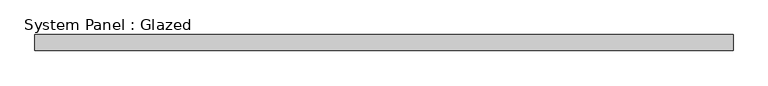
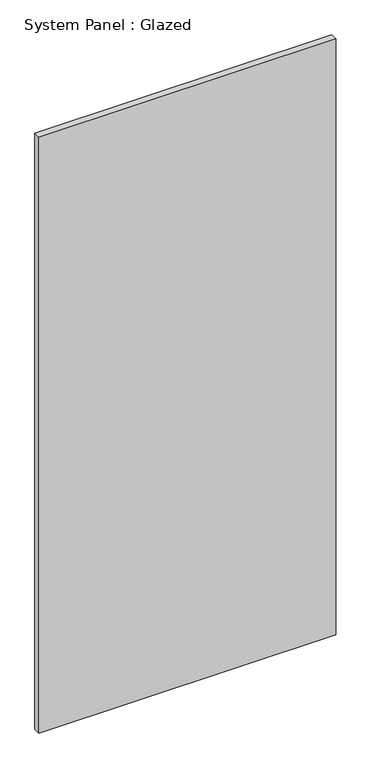
"""IFC4 building model written with IfcOpenShell, lengths in millimetres: plate geometry, System Panel : Glazed."""

from ifc_helpers import new_model, si_unit, origin, origin_with_axes, place, context, project, spatial, polyline, outline, extrude, source, transform, mapped, element, save


def system_panel_glazed_87980334(model_context):
    return source(origin(), model_context, "Body", "SweptSolid", [
        extrude(outline(polyline([(552.4499999, 19.05), (-552.4499999, 19.05), (-552.4499999, 44.45), (552.4499999, 44.45), (552.4499999, 19.05)])), origin_with_axes(), (0.0, 0.0, 1.0), 2343.15),
    ])


if __name__ == "__main__":
    model = new_model("IFC4")
    model_context = context("Model", 3, world=origin())
    ifc_project = project(units=[si_unit("LENGTHUNIT", "METRE", prefix="MILLI")], contexts=[model_context])
    site = spatial("IfcSite", under=ifc_project)
    building = spatial("IfcBuilding", under=site)
    placement = place(None, origin())
    system_panel_glazed_shape = system_panel_glazed_87980334(model_context)
    element("IfcPlate", 1, ObjectType="System Panel : Glazed", at=placement, inside=building, context=model_context, shape_type="MappedRepresentation", body=[
        mapped(system_panel_glazed_shape, transform((0.0, 0.0, 0.0), x_axis=(1.0, 0.0, 0.0), y_axis=(0.0, 1.0, 0.0), z_axis=(0.0, 0.0, 1.0))),
    ])
    save(model, "model.ifc")

# Revit data of these elements
# Type "System Panel : Glazed"
#   Construction Type Id = "GSP4R"
#   Analytic Construction = "1/8 in Pilkington single glazing"
#   Visual Light Transmittance = 0.9
#   Solar Heat Gain Coefficient = 0.86
#   Heat Transfer Coefficient (U) = 1.18115 BTU/(h·ft²·°F)
#   Define Thermal Properties by = 1
# Element 1 (IfcPlate, "System Panel : Glazed")
#   Materials on its faces: "glass panel 223"
# Materials
#   "glass panel 223": class "Generic", colour RGB 120 120 120, transparency 0, Cost = 0
